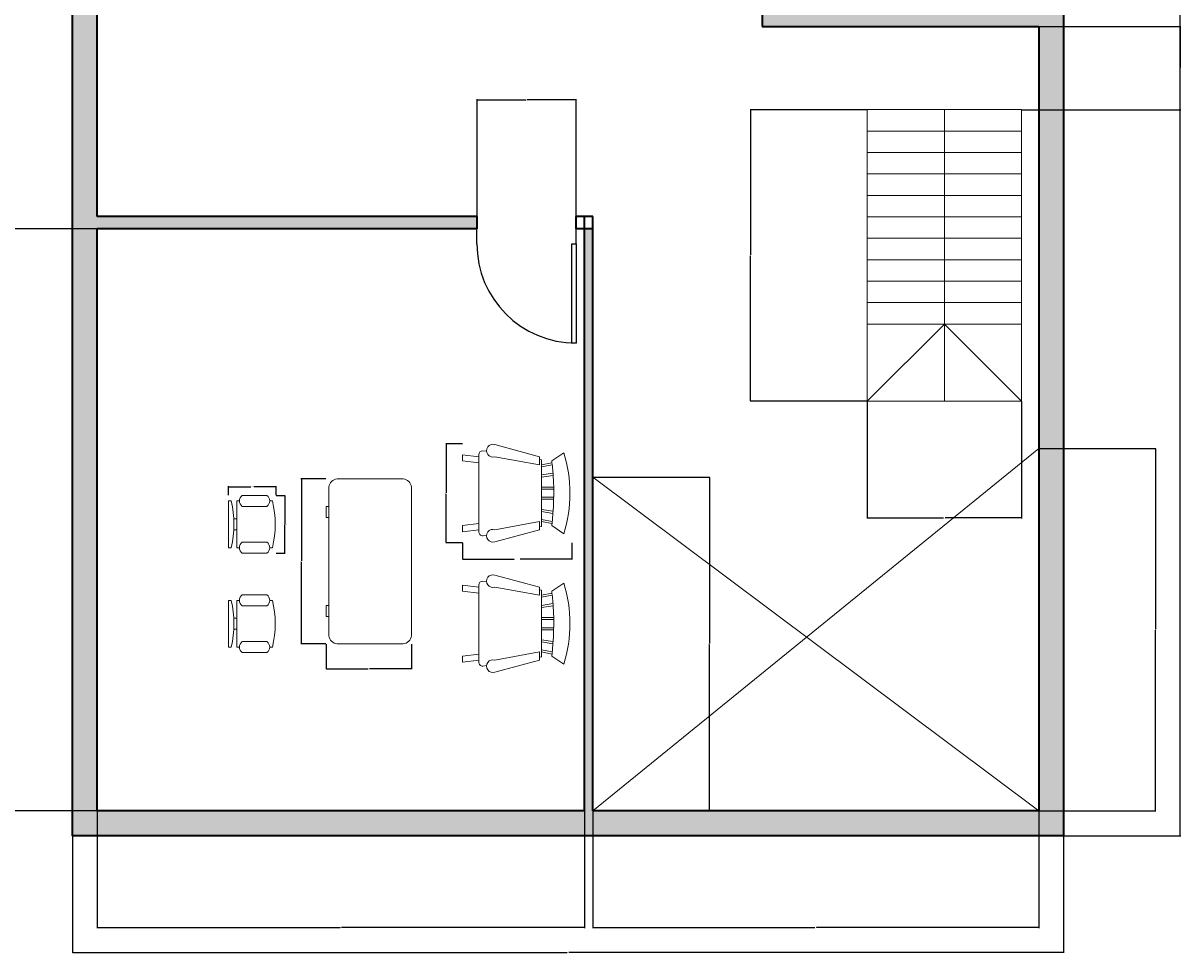
# Model space of a CAD drawing. Units: inches. Extents: x 1563 to 2428, y 777 to 1464.
# Tile 9 of 11: x 2007 to 2428, y 777 to 1115. Entities that reach past the tile are written whole.
import ezdxf

# ---------------------------------------------------------------- set-up
doc = ezdxf.new("R2010")
doc.units = ezdxf.units.IN
for name, color, linetype, lineweight in [('A-ANNO-DIMS', 2, 'Continuous', 18), ('A-DOOR', 4, 'Continuous', 25), ('A-FLOR-OPEN', 8, 'Continuous', 13), ('A-FLOR-STRS', 7, 'Continuous', 18), ('A-FURN', 9, 'Continuous', 18), ('A-WALL', 7, 'Continuous', 35), ('A-WALL-PATT', 8, 'Continuous', 13)]:
    doc.layers.add(name, color=color, linetype=linetype, lineweight=lineweight)
doc.styles.get("Standard").update_dxf_attribs({"font": 'arial.ttf'})
doc.dimstyles.get("Standard").update_dxf_attribs({"dimtxt": 0.18, "dimasz": 0.18, "dimexe": 0.18, "dimexo": 0.0625, "dimgap": 0.09, "dimtad": 0, "dimtih": 1, "dimtoh": 1, "dimdec": 4, "dimzin": 0, "dimdsep": 46, "dimtxsty": 'Standard', "dimcen": 0.09, "dimadec": 0, "dimazin": 0, "dimtfac": 1, "dimtdec": 4, "dimtofl": 0, "dimtmove": 0, "dimatfit": 3, "dimfxl": 1, "dimtolj": 1, "dimtzin": 0, "dimarcsym": 0})

# ---------------------------------------------------------------- blocks, each defined once
blk = doc.blocks.new('*U4')
for p, q in [((0, 0), (0, -6)), ((40, 0), (40, -6))]:
    blk.add_line(p, q)
blk.add_lwpolyline([(0, 0), (0, 40), (1.75, 40), (1.75, 0)], close=True)
blk.add_arc((0, 0), 40, 0, 90)
blk = doc.blocks.new('Chair - Desk')
for p, q in [((-8.5, 0), (-8.5, -1)), ((-8.5, 0), (8.5, 0)), ((8.5, 0), (8.5, -1)), ((-8.5, -3), (-8.5, -4)), ((-8.5, -3), (8.5, -3)), ((-2, -3), (-2, -1.9355)), ((2, -1.9576), (2, -3)), ((8.5, -3), (8.5, -4)), ((-10.5, -5), (-10.5, -14)), ((-6.5, -14), (-6.5, -5)), ((6.5, -5), (6.5, -14)), ((10.5, -14), (10.5, -5)), ((-8.5, -15), (-8.5, -16)), ((8.5, -15), (8.5, -16))]:
    blk.add_line(p, q)
for centre, radius, start, end in [((-8.5, -6.5), 2.5, 36.8699, 143.1301), ((0, 34.625), 36.625, 256.5803, 283.4197), ((8.5, -6.5), 2.5, 36.8699, 143.1301), ((-8.5, -12.5), 2.5, 216.8699, 323.1301), ((0, 19.625), 36.625, 256.5803, 283.4197), ((8.5, -12.5), 2.5, 216.8699, 323.1301)]:
    blk.add_arc(centre, radius, start, end)
blk = doc.blocks.new('Chair - Rocking')
for p, q in [((-8, -4.5), (-10, -1.5)), ((8, -4.5), (10, -1.5)), ((-7.5, -4.5), (-7, -7)), ((-6.5, -7), (-7.02225, -4.43)), ((-4.5, -7), (-4.96674, -4.19951)), ((-4, -7), (-4.40532, -4.16272)), ((-1.5, -4.05012), (-1.5, -7)), ((-1, -7), (-1, -4.05012)), ((1, -7), (1, -4.04655)), ((1.5, -4.05012), (1.5, -7)), ((4, -7), (4.40187, -4.18694)), ((4.5, -7), (4.96761, -4.19437)), ((6.5, -7), (7, -4.4057)), ((7.5, -4.5), (7, -7)), ((-9, -7.5), (-12, -18.49999)), ((-7, -7.5), (-9, -7.5)), ((-9, -18.49999), (-7, -7.5)), ((-8.23428, -6.99939), (-8.3093, -7.47958)), ((-8.23041, -7), (8.23915, -7)), ((7, -7.5), (9, -7.5)), ((9, -18.49999), (7, -7.5)), ((8.31071, -7.48854), (8.23449, -7.00073)), ((9, -7.5), (12, -18.49999)), ((-10.36644, -20.64523), (-10.5, -21.49999)), ((-9, -22.49999), (-9.5, -26.49999)), ((0, -22.49999), (-9.5, -22.49999)), ((-8, -26.49999), (-7.5, -22.49999)), ((0, -22.49999), (9.5, -22.49999)), ((8, -26.49999), (7.5, -22.49999)), ((9, -22.49999), (9.5, -26.49999)), ((10.5, -21.49999), (10.3575, -20.58798)), ((-9.5, -26.49999), (-8, -26.49999)), ((9.5, -26.49999), (8, -26.49999))]:
    blk.add_line(p, q)
for centre, radius, start, end in [((0, -34.08333), 34.08333, 72.93847, 107.0615), ((0, -68.25004), 64.25, 93.92211, 97.15267), ((0, -68.25004), 64.25, 82.84733, 93.92211), ((-10.5, -18.99999), 1.58114, 161.5651, 18.43495), ((10.5, -18.99999), 1.58114, 161.5651, 18.43495), ((-9.5, -21.49999), 1, 180, 270), ((9.5, -21.49999), 1, 270, 0)]:
    blk.add_arc(centre, radius, start, end)
blk = doc.blocks.new('Desk - 30 x 60 in.')
for p, q in [((-26.999995, 0), (26.999995, 0)), ((-29.999995, -27), (-29.999995, -3)), ((29.999995, -3), (29.999995, -27)), ((26.999995, -30), (-26.999995, -30)), ((-20.000005, -30), (-20.000005, -31)), ((-20.000005, -31), (-16.000005, -31)), ((-16.000005, -31), (-16.000005, -30)), ((15.999995, -31), (15.999995, -30)), ((19.999995, -31), (15.999995, -31)), ((19.999995, -30), (19.999995, -31))]:
    blk.add_line(p, q)
for centre, start, end in [((-26.499995, -3.5), 98.1301, 171.8699), ((26.499995, -3.5), 8.130102, 81.8699), ((-26.499995, -26.5), 188.1301, 261.8699), ((26.499995, -26.5), 278.1301, 351.8699)]:
    blk.add_arc(centre, 3.535534, start, end)
blk = doc.blocks.new('*D38')
at = {"layer": 'A-ANNO-DIMS', "color": 0, "lineweight": -2, "transparency": 16777216}
for p, q in [((2099.32, 942.97), (2102.59, 942.97)), ((2102.41, 942.79), (2102.41, 932.65)), ((2102.41, 922.15), (2102.41, 932.29)), ((2099.32, 921.97), (2102.59, 921.97))]:
    blk.add_line(p, q, dxfattribs=at)
at = {"layer": 'A-ANNO-DIMS', "color": 0, "transparency": 16777216}
for points in [[(2102.38, 942.79), (2102.44, 942.79), (2102.41, 942.97)], [(2102.38, 922.15), (2102.44, 922.15), (2102.41, 921.97)]]:
    blk.add_solid(points, dxfattribs=at)
at = {"layer": 'Defpoints', "color": 0, "transparency": 16777216}
for p in [(2099.26, 942.97), (2102.41, 942.97), (2099.26, 921.97)]:
    blk.add_point(p, dxfattribs=at)
at = {"layer": 'A-ANNO-DIMS', "color": 0, "transparency": 16777216, "insert": (2102.41, 932.47), "char_height": 0.18, "attachment_point": 5}
blk.add_mtext('\\A1;CHAIR 21 TYP.', dxfattribs=at)
blk = doc.blocks.new('*D39')
at = {"layer": 'A-ANNO-DIMS', "color": 0, "lineweight": -2, "transparency": 16777216}
for p, q in [((2081.93, 943.03), (2081.93, 946.3)), ((2099.26, 943.03), (2099.26, 946.3)), ((2082.11, 946.12), (2090.07, 946.12)), ((2099.08, 946.12), (2091.11, 946.12))]:
    blk.add_line(p, q, dxfattribs=at)
at = {"layer": 'A-ANNO-DIMS', "color": 0, "transparency": 16777216}
for points in [[(2082.11, 946.15), (2082.11, 946.09), (2081.93, 946.12)], [(2099.08, 946.15), (2099.08, 946.09), (2099.26, 946.12)]]:
    blk.add_solid(points, dxfattribs=at)
at = {"layer": 'Defpoints', "color": 0, "transparency": 16777216}
for p in [(2081.93, 946.12), (2081.93, 942.97), (2099.26, 942.97)]:
    blk.add_point(p, dxfattribs=at)
at = {"layer": 'A-ANNO-DIMS', "color": 0, "transparency": 16777216, "insert": (2090.59, 946.12), "char_height": 0.18, "attachment_point": 5}
blk.add_mtext('\\A1;17 TYP.', dxfattribs=at)
blk = doc.blocks.new('*D40')
at = {"layer": 'A-ANNO-DIMS', "color": 0, "lineweight": -2, "transparency": 16777216}
for p, q in [((2166.99, 925.71), (2166.99, 919.63)), ((2206.73, 925.71), (2206.73, 919.63)), ((2167.17, 919.81), (2185.76, 919.81)), ((2206.55, 919.81), (2187.96, 919.81))]:
    blk.add_line(p, q, dxfattribs=at)
at = {"layer": 'A-ANNO-DIMS', "color": 0, "transparency": 16777216}
for points in [[(2167.17, 919.84), (2167.17, 919.78), (2166.99, 919.81)], [(2206.55, 919.84), (2206.55, 919.78), (2206.73, 919.81)]]:
    blk.add_solid(points, dxfattribs=at)
at = {"layer": 'Defpoints', "color": 0, "transparency": 16777216}
for p in [(2166.99, 925.77), (2206.73, 925.77), (2206.73, 919.81)]:
    blk.add_point(p, dxfattribs=at)
at = {"layer": 'A-ANNO-DIMS', "color": 0, "transparency": 16777216, "insert": (2186.86, 919.81), "char_height": 0.18, "attachment_point": 5}
blk.add_mtext('\\A1;ROCKER 40 TYP.', dxfattribs=at)
blk = doc.blocks.new('*D41')
at = {"layer": 'A-ANNO-DIMS', "color": 0, "lineweight": -2, "transparency": 16777216}
for p, q in [((2166.93, 961.73), (2160.85, 961.73)), ((2161.03, 961.55), (2161.03, 943.94)), ((2161.03, 925.95), (2161.03, 943.57)), ((2166.93, 925.77), (2160.85, 925.77))]:
    blk.add_line(p, q, dxfattribs=at)
at = {"layer": 'A-ANNO-DIMS', "color": 0, "transparency": 16777216}
for points in [[(2161, 961.55), (2161.06, 961.55), (2161.03, 961.73)], [(2161, 925.95), (2161.06, 925.95), (2161.03, 925.77)]]:
    blk.add_solid(points, dxfattribs=at)
at = {"layer": 'Defpoints', "color": 0, "transparency": 16777216}
for p in [(2166.99, 961.73), (2161.03, 925.77), (2166.99, 925.77)]:
    blk.add_point(p, dxfattribs=at)
at = {"layer": 'A-ANNO-DIMS', "color": 0, "transparency": 16777216, "insert": (2161.03, 943.75), "char_height": 0.18, "attachment_point": 5}
blk.add_mtext('\\A1;36 TYP.', dxfattribs=at)
blk = doc.blocks.new('*D46')
at = {"layer": 'A-ANNO-DIMS', "color": 0, "lineweight": -2, "transparency": 16777216}
for p, q in [((2117.36, 948.97), (2108.25, 948.97)), ((2108.43, 948.79), (2108.43, 919.15)), ((2108.43, 889.15), (2108.43, 918.79)), ((2117.36, 888.97), (2108.25, 888.97))]:
    blk.add_line(p, q, dxfattribs=at)
at = {"layer": 'A-ANNO-DIMS', "color": 0, "transparency": 16777216}
for points in [[(2108.4, 948.79), (2108.46, 948.79), (2108.43, 948.97)], [(2108.4, 889.15), (2108.46, 889.15), (2108.43, 888.97)]]:
    blk.add_solid(points, dxfattribs=at)
at = {"layer": 'Defpoints', "color": 0, "transparency": 16777216}
for p in [(2117.43, 948.97), (2108.43, 888.97), (2117.43, 888.97)]:
    blk.add_point(p, dxfattribs=at)
at = {"layer": 'A-ANNO-DIMS', "color": 0, "transparency": 16777216, "insert": (2108.43, 918.97), "char_height": 0.18, "attachment_point": 5}
blk.add_mtext('\\A1;DESK 60', dxfattribs=at)
blk = doc.blocks.new('*D47')
at = {"layer": 'A-ANNO-DIMS', "color": 0, "lineweight": -2, "transparency": 16777216}
for p, q in [((2117.43, 888.91), (2117.43, 879.79)), ((2148.43, 888.91), (2148.43, 879.79)), ((2117.61, 879.97), (2132.72, 879.97)), ((2148.25, 879.97), (2133.13, 879.97))]:
    blk.add_line(p, q, dxfattribs=at)
at = {"layer": 'A-ANNO-DIMS', "color": 0, "transparency": 16777216}
for points in [[(2117.61, 880), (2117.61, 879.94), (2117.43, 879.97)], [(2148.25, 880), (2148.25, 879.94), (2148.43, 879.97)]]:
    blk.add_solid(points, dxfattribs=at)
at = {"layer": 'Defpoints', "color": 0, "transparency": 16777216}
for p in [(2117.43, 888.97), (2148.43, 888.97), (2148.43, 879.97)]:
    blk.add_point(p, dxfattribs=at)
at = {"layer": 'A-ANNO-DIMS', "color": 0, "transparency": 16777216, "insert": (2132.93, 879.97), "char_height": 0.18, "attachment_point": 5}
blk.add_mtext('\\A1;31', dxfattribs=at)
blk = doc.blocks.new('*D73')
at = {"layer": 'A-ANNO-DIMS', "color": 0, "lineweight": -2, "transparency": 16777216}
for p, q in [((2025.27, 819.26), (2025.27, 776.74)), ((2385.27, 819.26), (2385.27, 776.74)), ((2025.45, 776.92), (2204.98, 776.92)), ((2385.09, 776.92), (2205.56, 776.92))]:
    blk.add_line(p, q, dxfattribs=at)
at = {"layer": 'A-ANNO-DIMS', "color": 0, "transparency": 16777216}
for points in [[(2025.45, 776.95), (2025.45, 776.89), (2025.27, 776.92)], [(2385.09, 776.95), (2385.09, 776.89), (2385.27, 776.92)]]:
    blk.add_solid(points, dxfattribs=at)
at = {"layer": 'Defpoints', "color": 0, "transparency": 16777216}
for p in [(2025.27, 819.32), (2385.27, 819.32), (2385.27, 776.92)]:
    blk.add_point(p, dxfattribs=at)
at = {"layer": 'A-ANNO-DIMS', "color": 0, "transparency": 16777216, "insert": (2205.27, 776.92), "char_height": 0.18, "attachment_point": 5}
blk.add_mtext('\\A1;360', dxfattribs=at)
blk = doc.blocks.new('*D74')
at = {"layer": 'A-ANNO-DIMS', "color": 0, "lineweight": -2, "transparency": 16777216}
for p, q in [((2385.33, 1419.32), (2427.85, 1419.32)), ((2427.67, 1419.14), (2427.67, 1119.51)), ((2427.67, 819.5), (2427.67, 1119.14)), ((2385.33, 819.32), (2427.85, 819.32))]:
    blk.add_line(p, q, dxfattribs=at)
at = {"layer": 'A-ANNO-DIMS', "color": 0, "transparency": 16777216}
for points in [[(2427.64, 1419.14), (2427.7, 1419.14), (2427.67, 1419.32)], [(2427.64, 819.5), (2427.7, 819.5), (2427.67, 819.32)]]:
    blk.add_solid(points, dxfattribs=at)
at = {"layer": 'Defpoints', "color": 0, "transparency": 16777216}
for p in [(2385.27, 1419.32), (2385.27, 819.32), (2427.67, 819.32)]:
    blk.add_point(p, dxfattribs=at)
at = {"layer": 'A-ANNO-DIMS', "color": 0, "transparency": 16777216, "insert": (2427.67, 1119.32), "char_height": 0.18, "attachment_point": 5}
blk.add_mtext('\\A1;600', dxfattribs=at)
blk = doc.blocks.new('*D78')
at = {"layer": 'A-ANNO-DIMS', "color": 0, "lineweight": -2, "transparency": 16777216}
for p, q in [((2034.21, 1039.82), (1991.69, 1039.82)), ((1991.87, 1039.64), (1991.87, 934.26)), ((1991.87, 828.5), (1991.87, 933.89)), ((2034.21, 828.32), (1991.69, 828.32))]:
    blk.add_line(p, q, dxfattribs=at)
at = {"layer": 'A-ANNO-DIMS', "color": 0, "transparency": 16777216}
for points in [[(1991.84, 1039.64), (1991.9, 1039.64), (1991.87, 1039.82)], [(1991.84, 828.5), (1991.9, 828.5), (1991.87, 828.32)]]:
    blk.add_solid(points, dxfattribs=at)
at = {"layer": 'Defpoints', "color": 0, "transparency": 16777216}
for p in [(1991.87, 1039.82), (2034.27, 1039.82), (2034.27, 828.32)]:
    blk.add_point(p, dxfattribs=at)
at = {"layer": 'A-ANNO-DIMS', "color": 0, "transparency": 16777216, "insert": (1991.87, 934.07), "char_height": 0.18, "attachment_point": 5}
blk.add_mtext('\\A1;211.5', dxfattribs=at)
blk = doc.blocks.new('*D79')
at = {"layer": 'A-ANNO-DIMS', "color": 0, "lineweight": -2, "transparency": 16777216}
for p, q in [((2034.27, 828.26), (2034.27, 785.74)), ((2211.27, 828.26), (2211.27, 785.74)), ((2034.45, 785.92), (2122.49, 785.92)), ((2211.09, 785.92), (2123.05, 785.92))]:
    blk.add_line(p, q, dxfattribs=at)
at = {"layer": 'A-ANNO-DIMS', "color": 0, "transparency": 16777216}
for points in [[(2034.45, 785.95), (2034.45, 785.89), (2034.27, 785.92)], [(2211.09, 785.95), (2211.09, 785.89), (2211.27, 785.92)]]:
    blk.add_solid(points, dxfattribs=at)
at = {"layer": 'Defpoints', "color": 0, "transparency": 16777216}
for p in [(2034.27, 828.32), (2211.27, 828.32), (2034.27, 785.92)]:
    blk.add_point(p, dxfattribs=at)
at = {"layer": 'A-ANNO-DIMS', "color": 0, "transparency": 16777216, "insert": (2122.77, 785.92), "char_height": 0.18, "attachment_point": 5}
blk.add_mtext('\\A1;177', dxfattribs=at)
blk = doc.blocks.new('*D80')
at = {"layer": 'A-ANNO-DIMS', "color": 0, "lineweight": -2, "transparency": 16777216}
for p, q in [((2214.27, 828.26), (2214.27, 785.74)), ((2376.27, 828.26), (2376.27, 785.74)), ((2214.45, 785.92), (2294.99, 785.92)), ((2376.09, 785.92), (2295.55, 785.92))]:
    blk.add_line(p, q, dxfattribs=at)
at = {"layer": 'A-ANNO-DIMS', "color": 0, "transparency": 16777216}
for points in [[(2214.45, 785.95), (2214.45, 785.89), (2214.27, 785.92)], [(2376.09, 785.95), (2376.09, 785.89), (2376.27, 785.92)]]:
    blk.add_solid(points, dxfattribs=at)
at = {"layer": 'Defpoints', "color": 0, "transparency": 16777216}
for p in [(2214.27, 828.32), (2376.27, 828.32), (2214.27, 785.92)]:
    blk.add_point(p, dxfattribs=at)
at = {"layer": 'A-ANNO-DIMS', "color": 0, "transparency": 16777216, "insert": (2295.27, 785.92), "char_height": 0.18, "attachment_point": 5}
blk.add_mtext('\\A1;162', dxfattribs=at)
blk = doc.blocks.new('*D83')
at = {"layer": 'A-ANNO-DIMS', "color": 0, "lineweight": -2, "transparency": 16777216}
for p, q in [((2313.98, 977.1), (2313.98, 934.59)), ((2370.07, 977.1), (2370.07, 934.59)), ((2314.16, 934.77), (2341.72, 934.77)), ((2369.89, 934.77), (2342.33, 934.77))]:
    blk.add_line(p, q, dxfattribs=at)
at = {"layer": 'A-ANNO-DIMS', "color": 0, "transparency": 16777216}
for points in [[(2314.16, 934.8), (2314.16, 934.74), (2313.98, 934.77)], [(2369.89, 934.8), (2369.89, 934.74), (2370.07, 934.77)]]:
    blk.add_solid(points, dxfattribs=at)
at = {"layer": 'Defpoints', "color": 0, "transparency": 16777216}
for p in [(2313.98, 977.17), (2370.07, 977.17), (2313.98, 934.77)]:
    blk.add_point(p, dxfattribs=at)
at = {"layer": 'A-ANNO-DIMS', "color": 0, "transparency": 16777216, "insert": (2342.03, 934.77), "char_height": 0.18, "attachment_point": 5}
blk.add_mtext('\\A1;56.1', dxfattribs=at)
blk = doc.blocks.new('*D84')
at = {"layer": 'A-ANNO-DIMS', "color": 0, "lineweight": -2, "transparency": 16777216}
for p, q in [((2313.92, 1083.12), (2271.4, 1083.12)), ((2271.58, 1082.94), (2271.58, 1030.33)), ((2271.58, 977.35), (2271.58, 1029.96)), ((2313.92, 977.17), (2271.4, 977.17))]:
    blk.add_line(p, q, dxfattribs=at)
at = {"layer": 'A-ANNO-DIMS', "color": 0, "transparency": 16777216}
for points in [[(2271.55, 1082.94), (2271.61, 1082.94), (2271.58, 1083.12)], [(2271.55, 977.35), (2271.61, 977.35), (2271.58, 977.17)]]:
    blk.add_solid(points, dxfattribs=at)
at = {"layer": 'Defpoints', "color": 0, "transparency": 16777216}
for p in [(2271.58, 1083.12), (2313.98, 1083.12), (2313.98, 977.17)]:
    blk.add_point(p, dxfattribs=at)
at = {"layer": 'A-ANNO-DIMS', "color": 0, "transparency": 16777216, "insert": (2271.58, 1030.15), "char_height": 0.18, "attachment_point": 5}
blk.add_mtext('\\A1;105.96', dxfattribs=at)
blk = doc.blocks.new('*D85')
at = {"layer": 'A-ANNO-DIMS', "color": 0, "lineweight": -2, "transparency": 16777216}
for p, q in [((2376.33, 1113.32), (2427.85, 1113.32)), ((2427.67, 1113.14), (2427.67, 1098.41)), ((2427.67, 1083.3), (2427.67, 1098.04)), ((2370.14, 1083.12), (2427.85, 1083.12))]:
    blk.add_line(p, q, dxfattribs=at)
at = {"layer": 'A-ANNO-DIMS', "color": 0, "transparency": 16777216}
for points in [[(2427.64, 1113.14), (2427.7, 1113.14), (2427.67, 1113.32)], [(2427.64, 1083.3), (2427.7, 1083.3), (2427.67, 1083.12)]]:
    blk.add_solid(points, dxfattribs=at)
at = {"layer": 'Defpoints', "color": 0, "transparency": 16777216}
for p in [(2376.27, 1113.32), (2427.67, 1113.32), (2370.07, 1083.12)]:
    blk.add_point(p, dxfattribs=at)
at = {"layer": 'A-ANNO-DIMS', "color": 0, "transparency": 16777216, "insert": (2427.67, 1098.22), "char_height": 0.18, "attachment_point": 5}
blk.add_mtext('\\A1;30.2', dxfattribs=at)
blk = doc.blocks.new('*D88')
at = {"layer": 'A-ANNO-DIMS', "color": 0, "lineweight": -2, "transparency": 16777216}
for p, q in [((2172.27, 1044.39), (2172.27, 1086.9)), ((2172.45, 1086.72), (2190.05, 1086.72)), ((2208.09, 1086.72), (2190.49, 1086.72)), ((2208.27, 1044.39), (2208.27, 1086.9))]:
    blk.add_line(p, q, dxfattribs=at)
at = {"layer": 'A-ANNO-DIMS', "color": 0, "transparency": 16777216}
for points in [[(2172.45, 1086.75), (2172.45, 1086.69), (2172.27, 1086.72)], [(2208.09, 1086.75), (2208.09, 1086.69), (2208.27, 1086.72)]]:
    blk.add_solid(points, dxfattribs=at)
at = {"layer": 'Defpoints', "color": 0, "transparency": 16777216}
for p in [(2208.27, 1086.72), (2172.27, 1044.32), (2208.27, 1044.32)]:
    blk.add_point(p, dxfattribs=at)
at = {"layer": 'A-ANNO-DIMS', "color": 0, "transparency": 16777216, "insert": (2190.27, 1086.72), "char_height": 0.18, "attachment_point": 5}
blk.add_mtext('\\A1;36', dxfattribs=at)
blk = doc.blocks.new('*D90')
at = {"layer": 'A-ANNO-DIMS', "color": 0, "lineweight": -2, "transparency": 16777216}
for p, q in [((2376.33, 960.02), (2418.85, 960.02)), ((2418.67, 959.84), (2418.67, 894.35)), ((2418.67, 828.5), (2418.67, 893.99)), ((2376.33, 828.32), (2418.85, 828.32))]:
    blk.add_line(p, q, dxfattribs=at)
at = {"layer": 'A-ANNO-DIMS', "color": 0, "transparency": 16777216}
for points in [[(2418.64, 959.84), (2418.7, 959.84), (2418.67, 960.02)], [(2418.64, 828.5), (2418.7, 828.5), (2418.67, 828.32)]]:
    blk.add_solid(points, dxfattribs=at)
at = {"layer": 'Defpoints', "color": 0, "transparency": 16777216}
for p in [(2376.27, 960.02), (2376.27, 828.32), (2418.67, 828.32)]:
    blk.add_point(p, dxfattribs=at)
at = {"layer": 'A-ANNO-DIMS', "color": 0, "transparency": 16777216, "insert": (2418.67, 894.17), "char_height": 0.18, "attachment_point": 5}
blk.add_mtext('\\A1;131.7', dxfattribs=at)
blk = doc.blocks.new('*D91')
at = {"layer": 'A-ANNO-DIMS', "color": 0, "lineweight": -2, "transparency": 16777216}
for p, q in [((2214.33, 949.62), (2256.85, 949.62)), ((2256.67, 949.44), (2256.67, 889.15)), ((2256.67, 828.5), (2256.67, 888.79)), ((2214.33, 828.32), (2256.85, 828.32))]:
    blk.add_line(p, q, dxfattribs=at)
at = {"layer": 'A-ANNO-DIMS', "color": 0, "transparency": 16777216}
for points in [[(2256.64, 949.44), (2256.7, 949.44), (2256.67, 949.62)], [(2256.64, 828.5), (2256.7, 828.5), (2256.67, 828.32)]]:
    blk.add_solid(points, dxfattribs=at)
at = {"layer": 'Defpoints', "color": 0, "transparency": 16777216}
for p in [(2214.27, 949.62), (2214.27, 828.32), (2256.67, 828.32)]:
    blk.add_point(p, dxfattribs=at)
at = {"layer": 'A-ANNO-DIMS', "color": 0, "transparency": 16777216, "insert": (2256.67, 888.97), "char_height": 0.18, "attachment_point": 5}
blk.add_mtext('\\A1;121.3', dxfattribs=at)

msp = doc.modelspace()

# ---------------------------------------------------------------- hatches: boundary and pattern name
at = {"layer": 'A-WALL-PATT'}
h = msp.add_hatch(color=256, dxfattribs=at)
h.dxf.hatch_style = 1
h.paths.add_polyline_path([(2385.27, 1419.324), (2025.27, 1419.324), (2025.27, 819.324), (2385.27, 819.324)])
h.paths.add_polyline_path([(2034.27, 1410.324), (2112.27, 1410.324), (2112.27, 1257.324), (2116.77, 1257.324), (2116.77, 1410.324), (2376.27, 1410.324), (2376.27, 1218.324), (2158.77, 1218.324), (2158.77, 1213.824), (2376.27, 1213.824), (2376.27, 1117.824), (2280.27, 1117.824), (2280.27, 1174.824), (2275.77, 1174.824), (2275.77, 1113.324), (2376.27, 1113.324), (2376.27, 828.324), (2214.27, 828.324), (2214.27, 1039.824), (2211.27, 1039.824), (2211.27, 828.324), (2034.27, 828.324), (2034.27, 1039.824), (2172.27, 1039.824), (2172.27, 1044.324), (2034.27, 1044.324), (2034.27, 1136.044, -0.0910221), (2034.27, 1152.131), (2034.27, 1213.824), (2116.77, 1213.824), (2116.77, 1218.324), (2034.27, 1218.324)], flags=16)
h.paths.add_polyline_path([(2106.854, 1222.904), (2106.854, 1221.324), (2070.749, 1221.324), (2070.749, 1222.904)], flags=0)
h.paths.add_polyline_path([(2112.405, 1204.123), (2112.405, 1184.897), (2107.968, 1184.897), (2107.968, 1186.049), (2054.728, 1186.049), (2054.728, 1184.897), (2050.292, 1184.897), (2050.292, 1204.123, -0.1904762)], flags=0)
h.paths.add_polyline_path([(2090.222, 1205.162), (2090.222, 1200.143), (2072.475, 1200.143), (2072.475, 1205.162, -0.0496282)], flags=0)
h.paths.add_polyline_path([(2154.296, 1259.846), (2155.876, 1259.846), (2155.876, 1223.74), (2154.296, 1223.74)], flags=0)
h.paths.add_polyline_path([(2057.091, 1161.316), (2057.976, 1125.833), (2042.473, 1125.447, -0.2279232), (2041.588, 1160.929)], flags=0)
h.paths.add_polyline_path([(2070.302, 1156.728), (2114.669, 1156.728), (2114.669, 1134.544), (2070.302, 1134.544)], flags=0)
h.paths.add_polyline_path([(2098.463, 1153.659), (2098.693, 1153.693), (2098.873, 1153.74), (2099.01, 1153.799), (2099.116, 1153.868), (2099.197, 1153.947), (2099.257, 1154.032), (2099.297, 1154.124), (2099.319, 1154.22), (2099.325, 1154.317), (2099.317, 1154.416), (2099.296, 1154.513), (2099.264, 1154.608), (2099.223, 1154.698), (2099.175, 1154.784), (2099.152, 1154.822), (2099.024, 1155.024), (2098.98, 1155.1), (2098.886, 1155.294), (2098.952, 1155.577), (2099.204, 1155.752), (2099.49, 1155.809), (2099.811, 1155.818), (2100.249, 1155.79), (2100.399, 1155.774), (2100.143, 1155.797), (2099.922, 1155.811), (2099.732, 1155.816), (2099.57, 1155.811), (2099.432, 1155.797), (2099.315, 1155.774), (2099.215, 1155.742), (2099.129, 1155.7), (2099.057, 1155.651), (2099, 1155.594), (2098.956, 1155.532), (2098.926, 1155.465), (2098.91, 1155.395), (2098.907, 1155.322), (2098.919, 1155.249), (2098.944, 1155.175), (2098.98, 1155.1), (2099.024, 1155.024), (2099.073, 1154.947), (2099.124, 1154.867), (2099.239, 1154.68), (2099.35, 1154.353), (2099.273, 1154.02), (2099.025, 1153.78), (2098.599, 1153.668)], flags=0)
h.paths.add_polyline_path([(2102.466, 1148.582), (2102.722, 1148.584), (2102.944, 1148.598), (2103.134, 1148.624), (2103.296, 1148.662), (2103.434, 1148.711), (2103.551, 1148.771), (2103.651, 1148.84), (2103.737, 1148.919), (2103.808, 1149.01), (2103.864, 1149.116), (2103.904, 1149.241), (2103.928, 1149.386), (2103.936, 1149.554), (2103.926, 1149.749), (2103.898, 1149.974), (2103.852, 1150.229), (2103.791, 1150.508), (2103.719, 1150.804), (2103.639, 1151.108), (2103.554, 1151.411), (2103.468, 1151.707), (2103.384, 1151.986), (2103.306, 1152.242), (2103.192, 1152.613), (2103.109, 1152.925), (2103.073, 1153.241), (2103.204, 1153.522), (2103.537, 1153.75), (2103.928, 1153.83), (2104.287, 1153.815), (2104.697, 1153.701), (2104.827, 1153.641), (2104.593, 1153.73), (2104.384, 1153.788), (2104.194, 1153.819), (2104.014, 1153.826), (2103.845, 1153.813), (2103.688, 1153.781), (2103.546, 1153.733), (2103.421, 1153.671), (2103.313, 1153.597), (2103.225, 1153.514), (2103.158, 1153.425), (2103.114, 1153.329), (2103.091, 1153.226), (2103.088, 1153.111), (2103.103, 1152.981), (2103.134, 1152.832), (2103.179, 1152.662), (2103.237, 1152.466), (2103.306, 1152.242), (2103.384, 1151.986), (2103.468, 1151.707), (2103.554, 1151.411), (2103.639, 1151.108), (2103.719, 1150.804), (2103.831, 1150.346), (2103.921, 1149.846), (2103.94, 1149.459), (2103.881, 1149.105), (2103.667, 1148.829), (2103.373, 1148.68), (2103.05, 1148.605), (2102.609, 1148.576)], flags=0)
h.paths.add_polyline_path([(2105.563, 1146.7), (2105.82, 1146.77), (2106.045, 1146.848), (2106.242, 1146.934), (2106.417, 1147.025), (2106.572, 1147.121), (2106.714, 1147.219), (2106.846, 1147.317), (2107.065, 1147.484), (2107.307, 1147.648), (2107.597, 1147.802), (2107.932, 1147.921), (2108.322, 1147.996), (2108.777, 1148.019), (2109.297, 1147.991), (2109.852, 1147.914), (2110.415, 1147.796), (2110.559, 1147.756), (2110.278, 1147.825), (2109.995, 1147.884), (2109.715, 1147.933), (2109.438, 1147.971), (2109.169, 1147.998), (2108.91, 1148.012), (2108.664, 1148.014), (2108.433, 1148.002), (2108.22, 1147.977), (2108.024, 1147.939), (2107.843, 1147.889), (2107.675, 1147.83), (2107.519, 1147.76), (2107.372, 1147.683), (2107.234, 1147.599), (2107.102, 1147.509), (2106.974, 1147.415), (2106.747, 1147.242), (2106.488, 1147.063), (2106.146, 1146.883), (2105.705, 1146.729)], flags=0)
h.paths.add_polyline_path([(2114.376, 1144.033), (2114.426, 1144.021), (2114.436, 1144.02), (2114.305, 1144.051)], flags=0)
h.paths.add_polyline_path([(2242.564, 1401.056), (2376.27, 1401.056), (2376.27, 1300.776), (2242.564, 1300.776)], flags=0)
h.paths.add_polyline_path([(2326.799, 1326.18), (2352.203, 1326.18), (2352.203, 1387.685), (2374.265, 1387.685), (2374.265, 1352.922), (2352.203, 1352.922), (2352.203, 1348.91), (2374.265, 1348.91), (2374.265, 1314.147), (2348.86, 1314.147), (2348.86, 1322.838), (2326.799, 1300.776)], flags=0)
h.paths.add_polyline_path([(2313.978, 1083.124), (2342.025, 1083.124), (2370.073, 1083.124), (2370.073, 977.167), (2342.025, 977.167), (2313.978, 977.167)], flags=0)
h.paths.add_polyline_path([(1834.605, 1034.428), (1914.224, 1034.428), (1914.224, 1038.928), (1614.105, 1038.928), (1614.105, 1034.428), (1830.105, 1034.428), (1830.105, 830.428), (1834.605, 830.428)])

# ---------------------------------------------------------------- linework, layer by layer
at = {"layer": 'A-FLOR-OPEN'}
for p, q in [((2214.27, 828.324), (2376.27, 960.02)), ((2214.27, 949.621), (2376.27, 828.324))]:
    msp.add_line(p, q, dxfattribs=at)
at = {"layer": 'A-FLOR-STRS'}
msp.add_line((2342.025, 977.167), (2370.073, 977.167), dxfattribs=at)
msp.add_lwpolyline([(2342.025, 977.167), (2313.978, 977.167), (2342.025, 1005.214), (2370.073, 977.167), (2370.073, 1083.124), (2342.025, 1083.124)], close=True, dxfattribs=at)
for points in [[(2313.978, 977.167), (2313.978, 1083.124), (2342.025, 1083.124)], [(2370.073, 1075.333), (2342.025, 1075.333), (2313.978, 1075.333)], [(2370.073, 1067.542), (2342.025, 1067.542), (2313.978, 1067.542)], [(2370.073, 1059.751), (2342.025, 1059.751), (2313.978, 1059.751)], [(2370.073, 1051.96), (2342.025, 1051.96), (2313.978, 1051.96)], [(2370.073, 1044.169), (2342.025, 1044.169), (2313.978, 1044.169)], [(2370.073, 1036.378), (2342.025, 1036.378), (2313.978, 1036.378)], [(2370.073, 1028.587), (2342.025, 1028.587), (2313.978, 1028.587)], [(2370.073, 1020.796), (2342.025, 1020.796), (2313.978, 1020.796)], [(2370.073, 1013.005), (2342.025, 1013.005), (2313.978, 1013.005)], [(2313.978, 1005.214), (2342.025, 1005.214), (2370.073, 1005.214)]]:
    msp.add_lwpolyline(points, dxfattribs=at)
at = {"layer": 'A-WALL'}
for p, q in [((2034.27, 1044.324), (2034.27, 1213.824)), ((2275.77, 1174.824), (2275.77, 1113.324)), ((2275.77, 1113.324), (2376.27, 1113.324)), ((2376.27, 1113.324), (2376.27, 828.324)), ((2172.27, 1044.324), (2034.27, 1044.324)), ((2172.27, 1039.824), (2172.27, 1044.324)), ((2214.27, 1044.324), (2208.27, 1044.324)), ((2208.27, 1039.824), (2208.27, 1044.324)), ((2211.27, 828.324), (2211.27, 1044.324)), ((2214.27, 828.324), (2214.27, 1044.324)), ((2034.27, 828.324), (2034.27, 1039.824)), ((2172.27, 1039.824), (2034.27, 1039.824)), ((2214.27, 1039.824), (2208.27, 1039.824)), ((2211.27, 828.324), (2034.27, 828.324)), ((2376.27, 828.324), (2214.27, 828.324))]:
    msp.add_line(p, q, dxfattribs=at)
msp.add_lwpolyline([(2025.27, 1419.324), (2385.27, 1419.324), (2385.27, 819.324), (2025.27, 819.324)], close=True, dxfattribs=at)

# ---------------------------------------------------------------- block references
at = {"layer": 'A-DOOR', "xscale": 0.9026413098436022, "yscale": 0.9026413098436022, "zscale": 0.9026413098436022, "rotation": 180}
msp.add_blockref('*U4', (2208.27, 1034.408), dxfattribs=at)
at = {"layer": 'A-FURN', "xscale": 1.471697913848324, "yscale": 1.471697913848324, "zscale": 1.471697913848324, "rotation": 270}
for p in [(2205.993, 943.753), (2205.993, 896.368)]:
    msp.add_blockref('Chair - Rocking', p, dxfattribs=at)
at = {"layer": 'A-FURN'}
for name, p, rotation in [('Desk - 30 x 60 in.', (2148.426, 918.97), 270), ('Chair - Desk', (2081.926, 932.468), 90), ('Chair - Desk', (2081.926, 896.323), 90)]:
    msp.add_blockref(name, p, dxfattribs=dict(at, rotation=rotation))

# ---------------------------------------------------------------- dimensions: what is measured, and where the dimension line sits
at = {"layer": 'A-ANNO-DIMS'}
for base, p1, p2, angle, override, picture, middle in [((2427.67, 819.324), (2385.27, 1419.324), (2385.27, 819.324), 270, {"dimdec": 0, "dimlfac": 1, "dimrnd": 0, "dimzin": 0, "dimdsep": 46, "dimlunit": 2}, '*D74', (2427.67, 1119.324)), ((2427.67, 1113.324), (2370.073, 1083.124), (2376.27, 1113.324), 90, {"dimdec": 1, "dimlfac": 1, "dimrnd": 0, "dimzin": 0, "dimdsep": 46, "dimlunit": 2}, '*D85', (2427.67, 1098.224)), ((2271.578, 1083.124), (2313.978, 977.167), (2313.978, 1083.124), 90, {"dimdec": 2, "dimlfac": 1, "dimrnd": 0, "dimzin": 0, "dimdsep": 46, "dimlunit": 2}, '*D84', (2271.578, 1030.146)), ((1991.87, 1039.824), (2034.27, 828.324), (2034.27, 1039.824), 90, {"dimdec": 1, "dimlfac": 1, "dimrnd": 0, "dimzin": 0, "dimdsep": 46, "dimlunit": 2}, '*D78', (1991.87, 934.074)), ((2313.978, 934.767), (2370.073, 977.167), (2313.978, 977.167), 180, {"dimdec": 1, "dimlfac": 1, "dimrnd": 0, "dimzin": 0, "dimdsep": 46, "dimlunit": 2}, '*D83', (2342.025, 934.767)), ((2418.67, 828.324), (2376.27, 960.02), (2376.27, 828.324), 270, {"dimdec": 1, "dimlfac": 1, "dimrnd": 0, "dimzin": 0, "dimdsep": 46, "dimlunit": 2}, '*D90', (2418.67, 894.172)), ((2256.67, 828.324), (2214.27, 949.621), (2214.27, 828.324), 270, {"dimdec": 1, "dimlfac": 1, "dimrnd": 0, "dimzin": 0, "dimdsep": 46, "dimlunit": 2}, '*D91', (2256.67, 888.973)), ((2034.27, 785.924), (2211.27, 828.324), (2034.27, 828.324), 180, {"dimdec": 0, "dimlfac": 1, "dimrnd": 0, "dimzin": 0, "dimdsep": 46, "dimlunit": 2}, '*D79', (2122.77, 785.924)), ((2214.27, 785.924), (2376.27, 828.324), (2214.27, 828.324), 180, {"dimdec": 0, "dimlfac": 1, "dimrnd": 0, "dimzin": 0, "dimdsep": 46, "dimlunit": 2}, '*D80', (2295.27, 785.924))]:
    dim = msp.add_linear_dim(base=base, p1=p1, p2=p2, angle=angle, dimstyle='Standard', override=override, dxfattribs=at)
    dim.commit()
    dim.dimension.update_dxf_attribs({"geometry": picture, "text_midpoint": middle})
for base, p1, p2, picture, middle in [((2208.27, 1086.724), (2172.27, 1044.324), (2208.27, 1044.324), '*D88', (2190.27, 1086.724)), ((2148.426, 879.97), (2117.426, 888.97), (2148.426, 888.97), '*D47', (2132.926, 879.97)), ((2385.27, 776.924), (2025.27, 819.324), (2385.27, 819.324), '*D73', (2205.27, 776.924))]:
    dim = msp.add_linear_dim(base=base, p1=p1, p2=p2, dimstyle='Standard', override={"dimdec": 0, "dimlfac": 1, "dimrnd": 0, "dimzin": 0, "dimdsep": 46, "dimlunit": 2}, dxfattribs=at)
    dim.commit()
    dim.dimension.update_dxf_attribs({"geometry": picture, "text_midpoint": middle})
for base, p1, p2, angle, text, picture, middle in [((2161.033, 925.773), (2166.993, 961.734), (2166.993, 925.773), 270, '<> TYP.', '*D41', (2161.033, 943.753)), ((2081.926, 946.118), (2099.259, 942.968), (2081.926, 942.968), 180, '<> TYP.', '*D39', (2090.592, 946.118)), ((2108.426, 888.97), (2117.426, 948.97), (2117.426, 888.97), 270, 'DESK <>', '*D46', (2108.426, 918.97)), ((2102.409, 942.968), (2099.259, 921.968), (2099.259, 942.968), 90, 'CHAIR <> TYP.', '*D38', (2102.409, 932.468))]:
    dim = msp.add_linear_dim(base=base, p1=p1, p2=p2, angle=angle, text=text, dimstyle='Standard', override={"dimdec": 0, "dimlfac": 1, "dimrnd": 0, "dimzin": 0, "dimdsep": 46, "dimlunit": 2}, dxfattribs=at)
    dim.commit()
    dim.dimension.update_dxf_attribs({"geometry": picture, "text_midpoint": middle})
dim = msp.add_linear_dim(base=(2206.729, 919.812), p1=(2166.993, 925.773), p2=(2206.729, 925.773), text='ROCKER <> TYP.', dimstyle='Standard', override={"dimdec": 0, "dimlfac": 1, "dimrnd": 0, "dimzin": 0, "dimdsep": 46, "dimlunit": 2}, dxfattribs=at)
dim.commit()
dim.dimension.update_dxf_attribs({"geometry": '*D40', "text_midpoint": (2186.861, 919.812)})

doc.saveas('drawing.dxf')
